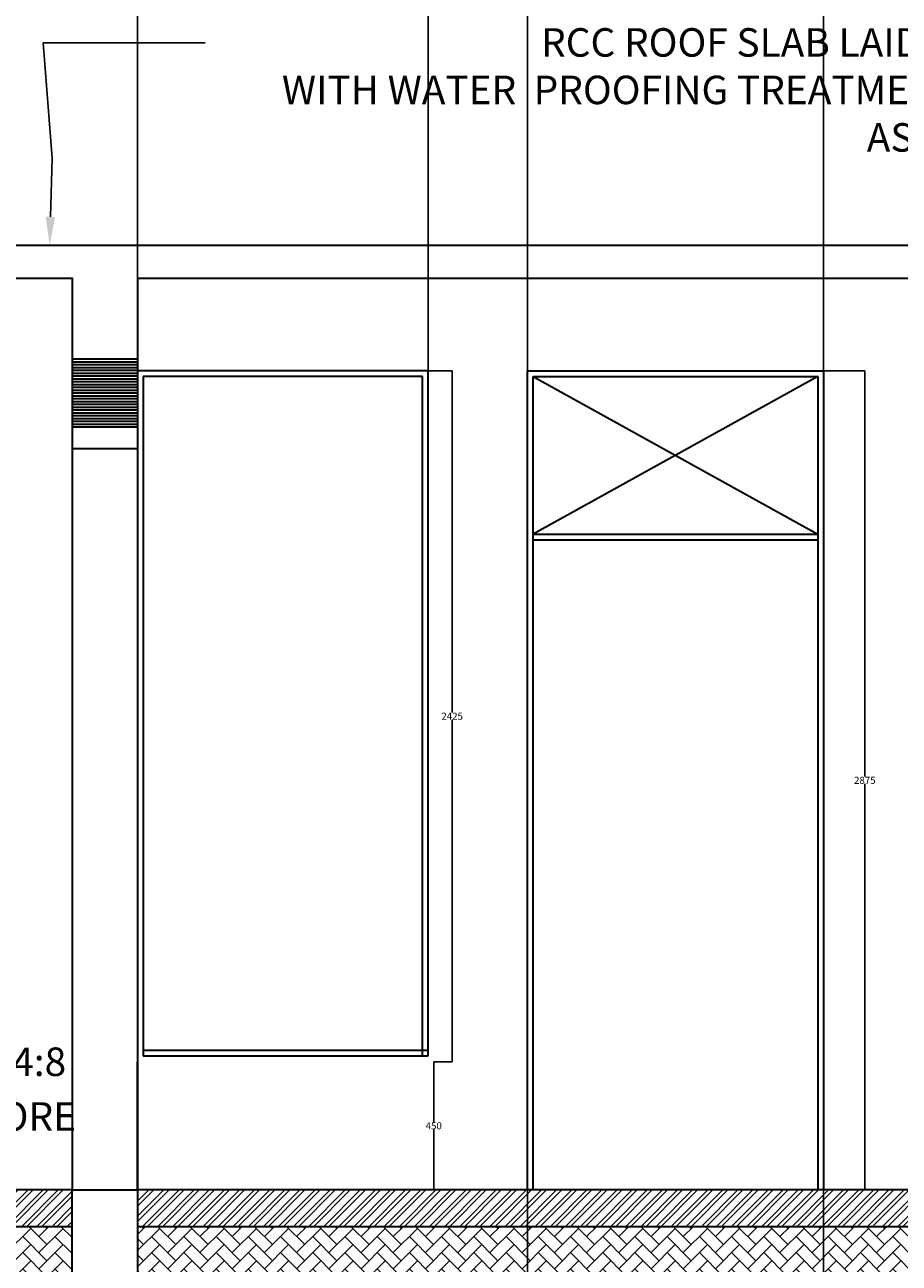
# Model space of a CAD drawing. Units: millimetres. Extents: x 1944 to 29915, y -10550 to 5909.
# Tile 13 of 24: x 16582 to 19652, y -6203 to -1857. Entities that reach past the tile are written whole.
import ezdxf
from ezdxf import colors
from ezdxf.entities.mleader import LeaderData, LeaderLine
from ezdxf.math import Vec2, Vec3

# ---------------------------------------------------------------- set-up
doc = ezdxf.new("R2010")
doc.units = ezdxf.units.MM
doc.header["$MEASUREMENT"] = 0
for name, color, linetype, lineweight in [('A-ANNO-DIMS', 2, 'Continuous', 18), ('A-ANNO-TEXT', 7, 'Continuous', 25), ('A-FLOR-PATT', 252, 'Continuous', 13), ('A-SECT', 7, 'Continuous', 35)]:
    doc.layers.add(name, color=color, linetype=linetype, lineweight=lineweight)
doc.styles.get("Standard").update_dxf_attribs({"font": 'arial.ttf'})
doc.dimstyles.get("Standard").update_dxf_attribs({"dimtxt": 25, "dimasz": 0.18, "dimexe": 0.18, "dimexo": 0.0625, "dimgap": 0.09, "dimtad": 0, "dimtih": 1, "dimtoh": 1, "dimdec": 0, "dimzin": 0, "dimdsep": 46, "dimtxsty": 'Standard', "dimcen": 0.09, "dimadec": 0, "dimazin": 0, "dimtfac": 1, "dimtdec": 0, "dimtofl": 0, "dimtmove": 0, "dimatfit": 3, "dimfxl": 1, "dimtolj": 1, "dimtzin": 0, "dimarcsym": 0})

# ---------------------------------------------------------------- blocks, each defined once
blk = doc.blocks.new('*D26')
at = {"layer": 'A-ANNO-DIMS', "color": 0, "lineweight": -2, "transparency": 16777216}
for p, q in [((18017.8, -5495.9), (18017.8, -5707.9)), ((18017.9, -5495.8), (18018, -5495.8)), ((18017.8, -5945.6), (18017.8, -5733.6)), ((18017.9, -5945.8), (18018, -5945.8))]:
    blk.add_line(p, q, dxfattribs=at)
at = {"layer": 'A-ANNO-DIMS', "color": 0, "transparency": 16777216}
for points in [[(18017.8, -5495.9), (18017.9, -5495.9), (18017.8, -5495.8)], [(18017.8, -5945.6), (18017.9, -5945.6), (18017.8, -5945.8)]]:
    blk.add_solid(points, dxfattribs=at)
at = {"layer": 'Defpoints', "color": 0, "transparency": 16777216}
for p in [(18017.8, -5495.8), (18017.8, -5945.8), (18017.8, -5945.8)]:
    blk.add_point(p, dxfattribs=at)
at = {"layer": 'A-ANNO-DIMS', "color": 0, "transparency": 16777216, "insert": (18017.8, -5720.8), "char_height": 25, "attachment_point": 5}
blk.add_mtext('\\A1;450', dxfattribs=at)
blk = doc.blocks.new('*D27')
at = {"layer": 'A-ANNO-DIMS', "color": 0, "lineweight": -2, "transparency": 16777216}
for p, q in [((17997.9, -3070.8), (18082.6, -3070.8)), ((18082.4, -3070.9), (18082.4, -4270.5)), ((18082.4, -5495.8), (18082.4, -4296.2)), ((18017.9, -5495.9), (18082.6, -5495.9))]:
    blk.add_line(p, q, dxfattribs=at)
at = {"layer": 'A-ANNO-DIMS', "color": 0, "transparency": 16777216}
for points in [[(18082.3, -3070.9), (18082.4, -3070.9), (18082.4, -3070.8)], [(18082.3, -5495.8), (18082.4, -5495.8), (18082.4, -5495.9)]]:
    blk.add_solid(points, dxfattribs=at)
at = {"layer": 'Defpoints', "color": 0, "transparency": 16777216}
for p in [(17997.8, -3070.8), (18082.4, -3070.8), (18017.9, -5495.9)]:
    blk.add_point(p, dxfattribs=at)
at = {"layer": 'A-ANNO-DIMS', "color": 0, "transparency": 16777216, "insert": (18082.4, -4283.3), "char_height": 25, "attachment_point": 5}
blk.add_mtext('\\A1;2425', dxfattribs=at)
blk = doc.blocks.new('*D28')
at = {"layer": 'A-ANNO-DIMS', "color": 0, "lineweight": -2, "transparency": 16777216}
for p, q in [((19366.7, -3070.8), (19531.7, -3070.8)), ((19531.5, -3070.9), (19531.5, -4495.4)), ((19531.5, -5945.6), (19531.5, -4521.1)), ((19366.7, -5945.8), (19531.7, -5945.8))]:
    blk.add_line(p, q, dxfattribs=at)
at = {"layer": 'A-ANNO-DIMS', "color": 0, "transparency": 16777216}
for points in [[(19531.5, -3070.9), (19531.6, -3070.9), (19531.5, -3070.8)], [(19531.5, -5945.6), (19531.6, -5945.6), (19531.5, -5945.8)]]:
    blk.add_solid(points, dxfattribs=at)
at = {"layer": 'Defpoints', "color": 0, "transparency": 16777216}
for p in [(19366.6, -3070.8), (19366.6, -5945.8), (19531.5, -5945.8)]:
    blk.add_point(p, dxfattribs=at)
at = {"layer": 'A-ANNO-DIMS', "color": 0, "transparency": 16777216, "insert": (19531.5, -4508.3), "char_height": 25, "attachment_point": 5}
blk.add_mtext('\\A1;2875', dxfattribs=at)
blk = doc.blocks.new('*D94')
at = {"layer": 'A-ANNO-DIMS', "color": 0, "lineweight": -2, "transparency": 16777216}
for p, q in [((16977.8, -3070.7), (16977.8, -395.6)), ((16978, -395.8), (17451.6, -395.8)), ((17997.6, -395.8), (17524, -395.8)), ((17997.8, -3070.7), (17997.8, -395.6))]:
    blk.add_line(p, q, dxfattribs=at)
at = {"layer": 'A-ANNO-DIMS', "color": 0, "transparency": 16777216}
for points in [[(16978, -395.7), (16978, -395.8), (16977.8, -395.8)], [(17997.6, -395.7), (17997.6, -395.8), (17997.8, -395.8)]]:
    blk.add_solid(points, dxfattribs=at)
at = {"layer": 'Defpoints', "color": 0, "transparency": 16777216}
for p in [(17997.8, -395.8), (16977.8, -3070.8), (17997.8, -3070.8)]:
    blk.add_point(p, dxfattribs=at)
at = {"layer": 'A-ANNO-DIMS', "color": 0, "transparency": 16777216, "insert": (17487.8, -395.8), "char_height": 25, "attachment_point": 5}
blk.add_mtext('\\A1;1020', dxfattribs=at)
blk = doc.blocks.new('*D95')
at = {"layer": 'A-ANNO-DIMS', "color": 0, "lineweight": -2, "transparency": 16777216}
for p, q in [((18346.6, -3070.7), (18346.6, -395.6)), ((18346.8, -395.8), (18830.4, -395.8)), ((19386.5, -395.8), (18902.8, -395.8)), ((19386.6, -3070.7), (19386.6, -395.6))]:
    blk.add_line(p, q, dxfattribs=at)
at = {"layer": 'A-ANNO-DIMS', "color": 0, "transparency": 16777216}
for points in [[(18346.8, -395.7), (18346.8, -395.8), (18346.6, -395.8)], [(19386.5, -395.7), (19386.5, -395.8), (19386.6, -395.8)]]:
    blk.add_solid(points, dxfattribs=at)
at = {"layer": 'Defpoints', "color": 0, "transparency": 16777216}
for p in [(19386.6, -395.8), (18346.6, -3070.8), (19386.6, -3070.8)]:
    blk.add_point(p, dxfattribs=at)
at = {"layer": 'A-ANNO-DIMS', "color": 0, "transparency": 16777216, "insert": (18866.6, -395.8), "char_height": 25, "attachment_point": 5}
blk.add_mtext('\\A1;1040', dxfattribs=at)
blk = doc.blocks.new('*D97')
at = {"layer": 'A-ANNO-DIMS', "color": 0, "lineweight": -2, "transparency": 16777216}
for p, q in [((16977.8, -5945.8), (16977.8, -10533.3)), ((18346.6, -5945.8), (18346.6, -10533.3)), ((16978, -10533.1), (17611.4, -10533.1)), ((18346.5, -10533.1), (17713.1, -10533.1))]:
    blk.add_line(p, q, dxfattribs=at)
at = {"layer": 'A-ANNO-DIMS', "color": 0, "transparency": 16777216}
for points in [[(16978, -10533.1), (16978, -10533.1), (16977.8, -10533.1)], [(18346.5, -10533.1), (18346.5, -10533.1), (18346.6, -10533.1)]]:
    blk.add_solid(points, dxfattribs=at)
at = {"layer": 'Defpoints', "color": 0, "transparency": 16777216}
for p in [(16977.8, -5945.8), (18346.6, -5945.8), (18346.6, -10533.1)]:
    blk.add_point(p, dxfattribs=at)
at = {"layer": 'A-ANNO-DIMS', "color": 0, "transparency": 16777216, "insert": (17662.2, -10533.1), "char_height": 25, "attachment_point": 5}
blk.add_mtext('\\A1;1368.8', dxfattribs=at)
blk = doc.blocks.new('*D98')
at = {"layer": 'A-ANNO-DIMS', "color": 0, "lineweight": -2, "transparency": 16777216}
for p, q in [((19386.6, -5945.8), (19386.6, -10533.3)), ((20755.4, -5945.8), (20755.4, -10533.3)), ((19386.8, -10533.1), (20020.2, -10533.1)), ((20755.3, -10533.1), (20121.9, -10533.1))]:
    blk.add_line(p, q, dxfattribs=at)
at = {"layer": 'A-ANNO-DIMS', "color": 0, "transparency": 16777216}
for points in [[(19386.8, -10533.1), (19386.8, -10533.1), (19386.6, -10533.1)], [(20755.3, -10533.1), (20755.3, -10533.1), (20755.4, -10533.1)]]:
    blk.add_solid(points, dxfattribs=at)
at = {"layer": 'Defpoints', "color": 0, "transparency": 16777216}
for p in [(19386.6, -5945.8), (20755.4, -5945.8), (20755.4, -10533.1)]:
    blk.add_point(p, dxfattribs=at)
at = {"layer": 'A-ANNO-DIMS', "color": 0, "transparency": 16777216, "insert": (20071, -10533.1), "char_height": 25, "attachment_point": 5}
blk.add_mtext('\\A1;1368.8', dxfattribs=at)

msp = doc.modelspace()

# ---------------------------------------------------------------- hatches: boundary and pattern name
at = {"layer": 'A-FLOR-PATT'}
h = msp.add_hatch(dxfattribs=at)
h.set_pattern_fill('ANSI32', color=256, scale=100)
h.paths.add_polyline_path([(16747.828, -5945.752), (12573.981, -5945.752), (12573.981, -6073.852), (16747.828, -6073.852)])
h = msp.add_hatch(dxfattribs=at)
h.set_pattern_fill('ANSI32', color=256, scale=100)
h.paths.add_polyline_path([(16977.828, -5945.752), (16977.828, -6073.852), (20755.45, -6073.852), (20755.45, -5945.752)])
h = msp.add_hatch(dxfattribs=at)
h.set_pattern_fill('AR-HBONE', color=256, scale=10)
h.paths.add_polyline_path([(12573.981, -6073.852), (12573.981, -6305.752), (16747.828, -6305.752), (16747.828, -6073.852)])
h = msp.add_hatch(dxfattribs=at)
h.set_pattern_fill('AR-HBONE', color=256, scale=10)
h.paths.add_polyline_path([(20755.45, -6073.852), (16977.828, -6073.852), (16977.828, -6305.752), (20755.45, -6305.752)])

# ---------------------------------------------------------------- linework, layer by layer
at = {"layer": 'A-SECT'}
for p, q in [((12343.981, -2630.752), (25389.297, -2630.752)), ((16977.828, -2745.752), (16977.828, -5945.752)), ((16977.828, -2745.752), (20755.45, -2745.752)), ((16977.828, -3030.752), (16747.828, -3030.752)), ((16977.828, -3040.684), (16747.828, -3040.684)), ((16977.828, -3030.752), (16977.828, -5495.752)), ((16977.828, -3050.616), (16747.828, -3050.616)), ((16977.828, -3060.549), (16747.828, -3060.549)), ((16977.828, -3070.481), (16747.828, -3070.481)), ((16977.828, -3080.414), (16747.828, -3080.414)), ((17997.828, -3070.752), (16977.828, -3070.752)), ((17997.828, -5475.752), (17997.828, -3070.752)), ((18346.639, -3070.752), (19386.639, -3070.752)), ((18346.639, -5945.752), (18346.639, -3070.752)), ((18346.639, -3070.752), (19386.639, -3070.752)), ((19386.639, -3070.752), (19386.639, -5945.752)), ((16977.828, -3090.346), (16747.828, -3090.346)), ((16977.828, -3100.279), (16747.828, -3100.279)), ((16977.828, -3110.211), (16747.828, -3110.211)), ((16977.828, -3120.143), (16747.828, -3120.143)), ((16997.828, -3090.752), (16997.828, -5475.752)), ((17977.828, -3090.752), (16997.828, -3090.752)), ((17977.828, -5475.752), (17977.828, -3090.752)), ((18366.639, -5945.752), (18366.639, -3090.752)), ((18366.639, -3090.752), (19366.639, -3090.752)), ((18366.639, -3090.752), (19366.639, -3644.839)), ((19366.639, -3090.752), (18366.639, -3644.839)), ((18366.639, -3644.839), (18366.639, -3090.752)), ((18366.639, -3090.752), (19366.639, -3090.752)), ((19366.639, -3090.752), (19366.639, -3644.839)), ((19366.639, -3090.752), (19366.639, -5945.752)), ((16977.828, -3130.076), (16747.828, -3130.076)), ((16977.828, -3140.008), (16747.828, -3140.008)), ((16977.828, -3149.941), (16747.828, -3149.941)), ((16977.828, -3159.873), (16747.828, -3159.873)), ((16977.828, -3169.806), (16747.828, -3169.806)), ((16977.828, -3179.738), (16747.828, -3179.738)), ((16977.828, -3189.67), (16747.828, -3189.67)), ((16977.828, -3199.603), (16747.828, -3199.603)), ((16977.828, -3209.535), (16747.828, -3209.535)), ((16977.828, -3219.468), (16747.828, -3219.468)), ((16977.828, -3229.4), (16747.828, -3229.4)), ((16977.828, -3239.333), (16747.828, -3239.333)), ((16977.828, -3249.265), (16747.828, -3249.265)), ((16977.828, -3259.198), (16747.828, -3259.198)), ((16977.828, -3269.13), (16747.828, -3269.13)), ((16977.828, -3345.404), (16747.828, -3345.404)), ((18366.639, -3644.839), (19366.639, -3644.839)), ((18366.639, -3664.839), (19366.639, -3664.839)), ((16997.828, -5455.752), (17997.828, -5455.752)), ((16997.828, -5475.752), (17997.828, -5475.752)), ((16977.828, -5945.752), (16977.828, -5495.752)), ((20755.45, -5945.752), (16977.828, -5945.752)), ((12573.981, -6073.852), (16747.828, -6073.852)), ((16977.828, -6073.852), (20755.45, -6073.852))]:
    msp.add_line(p, q, dxfattribs=at)
for points in [[(12573.981, -2745.752), (16747.828, -2745.752), (16747.828, -5945.752), (12573.981, -5945.752)], [(16747.828, -5945.752), (16977.828, -5945.752), (16977.828, -6305.752), (16747.828, -6305.752)]]:
    msp.add_lwpolyline(points, close=True, dxfattribs=at)

# ---------------------------------------------------------------- dimensions: what is measured, and where the dimension line sits
at = {"layer": 'A-ANNO-DIMS'}
for base, p1, p2, override, picture, middle in [((17997.828, -395.752), (16977.828, -3070.752), (17997.828, -3070.752), {"dimdec": 0, "dimlfac": 1, "dimrnd": 0, "dimzin": 0, "dimdsep": 46, "dimlunit": 2}, '*D94', (17487.828, -395.752)), ((19386.639, -395.752), (18346.639, -3070.752), (19386.639, -3070.752), {"dimdec": 0, "dimlfac": 1, "dimrnd": 0, "dimzin": 0, "dimdsep": 46, "dimlunit": 2}, '*D95', (18866.639, -395.752)), ((18346.639, -10533.115), (16977.828, -5945.752), (18346.639, -5945.752), {"dimdec": 1, "dimlfac": 1, "dimrnd": 0, "dimzin": 0, "dimdsep": 46, "dimlunit": 2}, '*D97', (17662.234, -10533.115)), ((20755.45, -10533.115), (19386.639, -5945.752), (20755.45, -5945.752), {"dimdec": 1, "dimlfac": 1, "dimrnd": 0, "dimzin": 0, "dimdsep": 46, "dimlunit": 2}, '*D98', (20071.044, -10533.115))]:
    dim = msp.add_linear_dim(base=base, p1=p1, p2=p2, dimstyle='Standard', override=override, dxfattribs=at)
    dim.commit()
    dim.dimension.update_dxf_attribs({"geometry": picture, "text_midpoint": middle})
for base, p1, p2, picture, middle in [((18082.374, -3070.752), (18017.858, -5495.932), (17997.828, -3070.752), '*D27', (18082.374, -4283.342)), ((19531.533, -5945.752), (19366.639, -3070.752), (19366.639, -5945.752), '*D28', (19531.533, -4508.252)), ((18017.828, -5945.752), (18017.828, -5495.752), (18017.828, -5945.752), '*D26', (18017.828, -5720.752))]:
    dim = msp.add_linear_dim(base=base, p1=p1, p2=p2, angle=90, dimstyle='Standard', override={"dimclrd": 0, "dimclre": 0, "dimclrt": 0}, dxfattribs=at)
    dim.commit()
    dim.dimension.update_dxf_attribs({"geometry": picture, "text_midpoint": middle})

# ---------------------------------------------------------------- leaders
at = {"layer": 'A-ANNO-TEXT'}
ml = msp.add_multileader_mtext('Standard', dxfattribs=at)
ml.set_content('RCC ROOF SLAB LAID TO SLOPE \\PWITH WATER  PROOFING TREATMENT ON TOP \\PAS SPECIFIED', color=256)
ml.set_leader_properties()
ml.build(insert=Vec2(0, 0))
ml.multileader.update_dxf_attribs({"dogleg_length": 568.936, "arrow_head_size": 100})
ctx = ml.context
ctx.base_point, ctx.char_height, ctx.arrow_head_size, ctx.landing_gap_size, ctx.plane_origin = Vec3(17215.618, -1919.582), 100, 100, 0.09, Vec3(17085.053, -2367.807)
ctx.text_align_type = 2
notes = []
notes.append((ctx, [(0, (1, 1, 0), (16646.682, -1919.582), (1, 0), 568.936, [(0, [(16669.038, -2630.752), (16677.34, -2324.48)], 0, [])])]))
ctx.mtext.insert, ctx.mtext.alignment, ctx.mtext.flow_direction = Vec3(20397.632, -1868.729), 3, 5
ml = msp.add_multileader_mtext('Standard', dxfattribs=at)
ml.set_content('7TH HARD PCC 1:4:8', color=256)
ml.set_leader_properties()
ml.build(insert=Vec2(0, 0))
ml.multileader.update_dxf_attribs({"dogleg_length": 568.936, "arrow_head_size": 100})
ctx = ml.context
ctx.base_point, ctx.char_height, ctx.arrow_head_size, ctx.landing_gap_size, ctx.plane_origin = Vec3(15357.883, -5496.91), 100, 100, 0.09, Vec3(14788.948, -5496.91)
ctx.text_align_type = 2
notes.append((ctx, [(0, (1, 1, 0), (14788.948, -5496.91), (1, 0), 568.936, [(0, [(14293.563, -6045.171), (14293.563, -5492.056)], 0, [])])]))
ctx.mtext.insert, ctx.mtext.alignment, ctx.mtext.flow_direction = Vec3(16727.073, -5446.057), 3, 5
ml = msp.add_multileader_mtext('Standard', dxfattribs=at)
ml.set_content('7TH .HARD CORE', color=256)
ml.set_leader_properties()
ml.build(insert=Vec2(0, 0))
ml.multileader.update_dxf_attribs({"dogleg_length": 568.936, "arrow_head_size": 100})
ctx = ml.context
ctx.base_point, ctx.char_height, ctx.arrow_head_size, ctx.landing_gap_size, ctx.plane_origin = Vec3(15595.87, -5688.802), 100, 100, 0.09, Vec3(15026.935, -5688.802)
ctx.text_align_type = 2
notes.append((ctx, [(0, (1, 1, 0), (15026.935, -5688.802), (1, 0), 568.936, [(0, [(14533.534, -6115.34), (14531.55, -5683.948)], 0, [])])]))
ctx.mtext.insert, ctx.mtext.alignment, ctx.mtext.flow_direction = Vec3(16761.649, -5637.949), 3, 5
for ctx, leaders in notes:
    for number, flags, end, landing, length, lines in leaders:
        leader = LeaderData()
        leader.index, (leader.has_last_leader_line, leader.has_dogleg_vector, leader.attachment_direction) = number, flags
        leader.last_leader_point, leader.dogleg_vector, leader.dogleg_length = Vec3(end), Vec3(landing), length
        for number, points, colour, breaks in lines:
            line = LeaderLine()
            line.index, line.vertices, line.color, line.breaks = number, Vec3.list(points), colors.encode_raw_color(colour), breaks
            leader.lines.append(line)
        ctx.leaders.append(leader)

doc.saveas('drawing.dxf')
